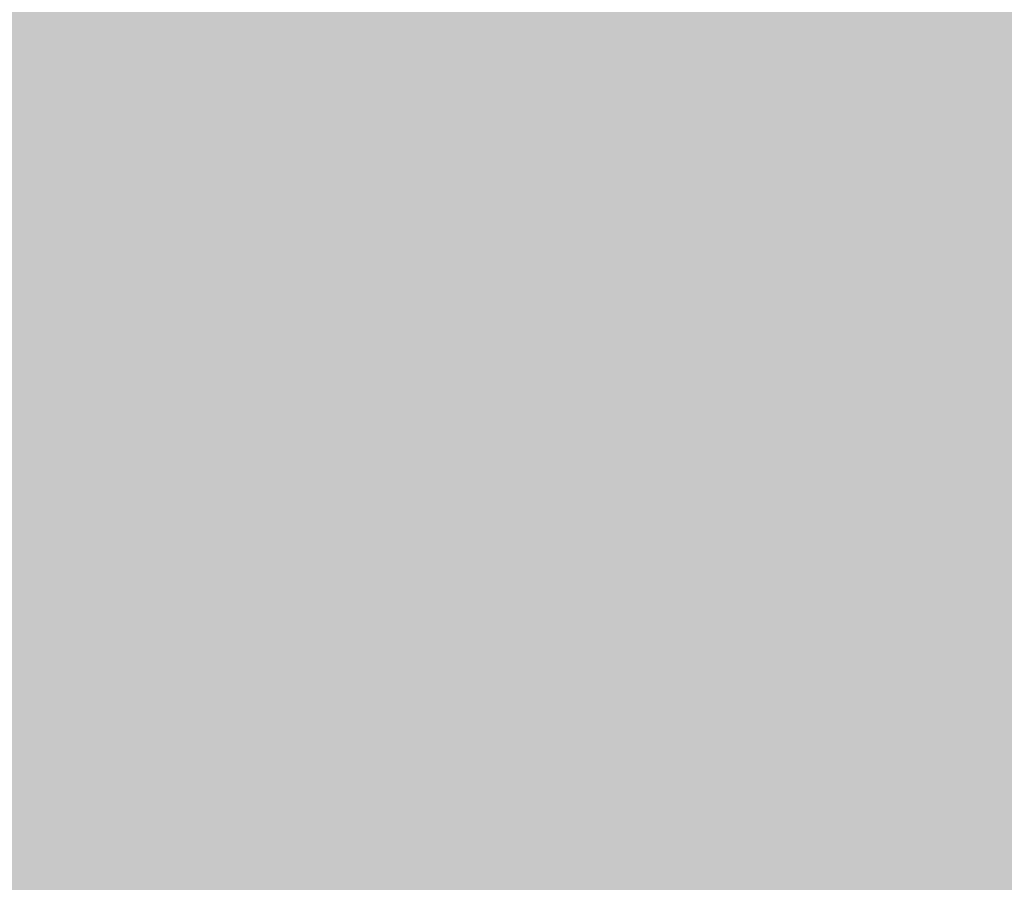
# Model space of a CAD drawing. Units: inches. Extents: x 2083 to 3317, y 1141 to 2115.
# Tile 149 of 256: x 3126.92826 to 3126.94671, y 1263.27402 to 1263.29018. Entities that reach past the tile are written whole.
import ezdxf

# ---------------------------------------------------------------- set-up
doc = ezdxf.new("R2010")
doc.units = ezdxf.units.IN
doc.layers.add('A-ANNO-DIMS', color=2, linetype='Continuous', lineweight=18)
doc.layers.add('A-WALL-PATT', color=251, linetype='Continuous', lineweight=13, true_color=0x636466)
doc.styles.get("Standard").update_dxf_attribs({"font": 'arial.ttf'})
doc.dimstyles.new('ISO-25', dxfattribs={"dimtxt": 12, "dimasz": 12, "dimexe": 1.25, "dimexo": 0.625, "dimtad": 1, "dimlunit": 3, "dimtxsty": 'Standard', "dimcen": 2.5, "dimadec": 0, "dimazin": 0, "dimtfac": 1, "dimtmove": 0, "dimatfit": 3, "dimfxl": 1, "dimarcsym": 0})

# ---------------------------------------------------------------- blocks, each defined once
blk = doc.blocks.new('*D26')
at = {"layer": 'A-ANNO-DIMS', "color": 0, "lineweight": -2, "transparency": 16777216}
for p, q in [((3088.985844, 1274.915092), (3088.985844, 1270.951963)), ((3111.240037, 1274.915092), (3111.240037, 1270.951963)), ((3076.985844, 1272.201963), (2840.262447, 1272.201963)), ((3111.240037, 1272.201963), (3088.985844, 1272.201963)), ((3123.240037, 1272.201963), (3135.240037, 1272.201963))]:
    blk.add_line(p, q, dxfattribs=at)
at = {"layer": 'A-ANNO-DIMS', "color": 0, "transparency": 16777216}
for points in [[(3076.985844, 1274.201963), (3076.985844, 1270.201963), (3088.985844, 1272.201963)], [(3123.240037, 1274.201963), (3123.240037, 1270.201963), (3111.240037, 1272.201963)]]:
    blk.add_solid(points, dxfattribs=at)
at = {"layer": 'Defpoints', "color": 0, "transparency": 16777216}
for p in [(3088.985844, 1275.540092), (3111.240037, 1275.540092), (3088.985844, 1272.201963)]:
    blk.add_point(p, dxfattribs=at)
at = {"layer": 'A-ANNO-DIMS', "color": 0, "transparency": 16777216, "insert": (2952.624146, 1279.031602), "char_height": 12, "attachment_point": 5}
blk.add_mtext('NIGHTSTAND 1\'-10 1/2" TYP.', dxfattribs=at)
blk = doc.blocks.new('*D27')
at = {"layer": 'A-ANNO-DIMS', "color": 0, "lineweight": -2, "transparency": 16777216}
for p, q in [((3114.578165, 1309.794285), (3114.578165, 1321.794285)), ((3111.865037, 1297.794285), (3115.828165, 1297.794285)), ((3114.578165, 1297.794285), (3114.578165, 1275.540092)), ((3111.865037, 1275.540092), (3115.828165, 1275.540092)), ((3114.578165, 1263.540092), (3114.578165, 1140.988591))]:
    blk.add_line(p, q, dxfattribs=at)
at = {"layer": 'A-ANNO-DIMS', "color": 0, "transparency": 16777216}
for points in [[(3112.578165, 1309.794285), (3116.578165, 1309.794285), (3114.578165, 1297.794285)], [(3112.578165, 1263.540092), (3116.578165, 1263.540092), (3114.578165, 1275.540092)]]:
    blk.add_solid(points, dxfattribs=at)
at = {"layer": 'Defpoints', "color": 0, "transparency": 16777216}
for p in [(3111.240037, 1297.794285), (3111.240037, 1275.540092), (3114.578165, 1275.540092)]:
    blk.add_point(p, dxfattribs=at)
at = {"layer": 'A-ANNO-DIMS', "color": 0, "transparency": 16777216, "insert": (3107.748527, 1196.264342), "char_height": 12, "attachment_point": 5, "rotation": 90}
blk.add_mtext('1\'-10 1/2" TYP.', dxfattribs=at)

msp = doc.modelspace()

# ---------------------------------------------------------------- hatches: boundary and pattern name
at = {"layer": 'A-WALL-PATT'}
h = msp.add_hatch(color=256, dxfattribs=at)
h.dxf.hatch_style = 1
h.paths.add_polyline_path([(3126.959783, 2020.76136), (2748.959783, 2020.76136), (2604.959783, 2020.76136), (2226.959783, 2020.76136), (2226.959783, 1702.76136), (2466.959783, 1702.76136), (2466.959783, 1582.76136), (2418.959783, 1582.76136), (2418.959783, 1477.76136), (2226.959783, 1477.76136), (2226.959783, 1263.26136), (2544.959783, 1263.26136), (2544.959783, 1411.76136), (2604.959783, 1411.76136), (2685.959783, 1411.76136), (2685.959783, 1420.76136), (2604.959783, 1420.76136), (2604.959783, 1573.76136), (2604.959783, 1702.76136), (2604.959783, 2011.76136), (2748.959783, 2011.76136), (2748.959783, 1702.76136), (2862.959783, 1702.76136), (2862.959783, 1621.76136), (2871.959783, 1621.76136), (2871.959783, 1702.76136), (2883.959783, 1702.76136), (2883.959783, 1706.939459, -0.026459), (2883.959783, 1711.76136), (2757.959783, 1711.76136), (2757.959783, 1807.76136), (2787.959783, 1807.76136), (2787.959783, 1812.26136), (2757.959783, 1812.26136), (2757.959783, 2011.76136), (2877.959783, 2011.76136), (2877.959783, 1812.26136), (2847.959783, 1812.26136), (2847.959783, 1807.76136), (2889.835742, 1807.76136), (2889.835742, 1812.26136), (2882.459783, 1812.26136), (2882.459783, 2011.76136), (3117.959783, 2011.76136), (3117.959783, 1812.26136), (2937.835742, 1812.26136), (2937.835742, 1807.76136), (2995.709783, 1807.76136), (2995.709783, 1796.117666), (3000.209783, 1796.117666), (3000.209783, 1807.76136), (3117.959783, 1807.76136), (3117.959783, 1711.76136), (3000.209783, 1711.76136), (3000.209783, 1760.117666), (2998.572705, 1760.117666, -0.020711), (2995.709783, 1760.117666), (2995.709783, 1711.76136), (2931.959783, 1711.76136), (2931.959783, 1702.76136), (3126.959783, 1702.76136)])
h.paths.add_polyline_path([(2471.459783, 2011.76136), (2471.459783, 1810.01136), (2462.716936, 1810.01136), (2462.716936, 1805.51136), (2505.959783, 1805.51136), (2505.959783, 1810.01136), (2475.959783, 1810.01136), (2475.959783, 2011.76136), (2595.959783, 2011.76136), (2595.959783, 1810.01136), (2565.959783, 1810.01136), (2565.959783, 1805.51136), (2595.959783, 1805.51136), (2595.959783, 1711.76136), (2235.959783, 1711.76136), (2235.959783, 1805.51136), (2353.709783, 1805.51136), (2353.709783, 1796.054162), (2358.209783, 1796.054162), (2358.209783, 1805.51136), (2414.716936, 1805.51136), (2414.716936, 1810.01136), (2235.959783, 1810.01136), (2235.959783, 2011.76136)], flags=16)
h.paths.add_polyline_path([(2270.204734, 1994.610008), (2270.204734, 1970.610008), (2246.204734, 1970.610008), (2246.204734, 1994.610008)], flags=0)
edge = h.paths.add_edge_path(flags=0)
edge.add_ellipse((2332.027391, 1899.798176), major_axis=(-3.042994, 3.042994), ratio=0.16825245, start_angle=-161.332166, end_angle=-156.307114, ccw=False)
edge.add_ellipse((2333.082037, 1898.74353), major_axis=(-1.054646, 1.054646), ratio=0.4535321, start_angle=-123.371019, end_angle=-94.159107)
edge = h.paths.add_edge_path(flags=0)
edge.add_ellipse((2332.027391, 1968.87629), major_axis=(3.042994, 3.042994), ratio=0.16825245, start_angle=18.667834, end_angle=23.692886)
edge.add_spline(control_points=[(2332.925596, 1970.691105), (2332.226768, 1970.3361), (2330.893709, 1969.658905), (2328.41308, 1970.932138), (2327.203934, 1967.748712), (2324.709596, 1969.955589), (2322.532822, 1967.012354), (2320.012846, 1971.295812), (2317.680308, 1968.157845), (2316.040526, 1967.102047), (2315.426904, 1966.809602)], knot_values=[0, 0, 0, 0, 2.267059, 4.324559, 6.685584, 8.878641, 11.121502, 14.300359, 17.755284, 19.732645, 19.732645, 19.732645, 19.732645], degree=3, periodic=0)
edge.add_ellipse((2332.027391, 1968.87629), major_axis=(3.042994, 3.042994), ratio=0.16825245, start_angle=18.667834, end_angle=23.692886, ccw=False)
edge.add_ellipse((2333.082037, 1969.930936), major_axis=(1.054646, 1.054646), ratio=0.4535321, start_angle=56.628981, end_angle=85.840893, ccw=False)
edge = h.paths.add_edge_path(flags=0)
edge.add_spline(control_points=[(2296.428287, 1967.987908), (2293.627804, 1965.336314), (2287.703624, 1959.727094), (2299.74386, 1949.995699), (2294.532591, 1935.668528), (2290.573228, 1920.603512), (2293.394124, 1909.973691), (2296.185407, 1904.966543)], knot_values=[0.099185, 0.099185, 0.099185, 0.099185, 0.345301, 0.619822, 0.982653, 1.386093, 1.810555, 1.810555, 1.810555, 1.810555], degree=3, periodic=0)
edge.add_spline(control_points=[(2296.185407, 1904.966543), (2297.383582, 1902.6193), (2298.000969, 1901.949312), (2298.55297, 1901.468155)], knot_values=[0.006246, 0.006246, 0.006246, 0.006246, 0.055476, 0.055476, 0.055476, 0.055476], degree=3, periodic=0)
edge.add_spline(control_points=[(2298.55297, 1901.468155), (2297.258612, 1900.923224), (2295.225294, 1900.232126), (2293.060229, 1900.614205), (2292.101423, 1900.788415), (2292.089578, 1900.790568)], knot_values=[0.312835, 0.312835, 0.312835, 0.312835, 0.40178, 0.474987, 0.475903, 0.475903, 0.475903, 0.475903], degree=3, periodic=0)
edge.add_arc((2292.793646, 1904.664109), 3.937008, 215.420897, 259.698179, ccw=False)
edge.add_spline(control_points=[(2289.585314, 1902.382304), (2289.476652, 1902.535087), (2289.36848, 1902.688035), (2289.260865, 1902.84117)], knot_values=[0.102872, 0.102872, 0.102872, 0.102872, 0.116896, 0.116896, 0.116896, 0.116896], degree=3, periodic=0)
edge.add_spline(control_points=[(2289.260865, 1902.84117), (2288.686604, 1902.550192), (2287.640048, 1902.019902), (2285.881337, 1901.873954), (2283.852972, 1901.504352), (2281.719987, 1899.710538), (2278.466991, 1899.492942), (2276.157136, 1901.883202), (2272.258953, 1899.804071), (2267.777605, 1901.843183), (2262.243882, 1900.184033), (2257.414927, 1901.782061), (2254.318374, 1900.72612), (2253.178285, 1900.337343)], knot_values=[0, 0, 0, 0, 1.907977, 3.477176, 5.261074, 7.972851, 11.680248, 13.717921, 16.939592, 22.789562, 27.502503, 33.595215, 37.145618, 37.145618, 37.145618, 37.145618], degree=3, periodic=0)
edge.add_line((2253.178285, 1900.337343), (2250.24424, 1902.84117))
edge.add_line((2250.24424, 1902.84117), (2250.24424, 1965.833296))
edge.add_line((2250.24424, 1965.833296), (2253.178285, 1968.337123))
edge.add_spline(control_points=[(2253.178285, 1968.337123), (2254.318374, 1967.948346), (2257.414927, 1966.892405), (2262.243882, 1968.490433), (2267.777605, 1966.831283), (2271.52673, 1968.537217), (2273.875914, 1967.828289), (2274.206701, 1967.727642)], knot_values=[0, 0, 0, 0, 0.09018, 0.244935, 0.364644, 0.513233, 0.537855, 0.537855, 0.537855, 0.537855], degree=3, periodic=0)
edge.add_arc((2274.352887, 1963.793349), 3.937008, 72.051134, 92.127949, ccw=False)
edge.add_arc((2281.296933, 1985.230003), 18.596298, 252.0511336, 288.5657217)
edge.add_arc((2292.316717, 1956.02888), 12.646081, 71.0267879, 113.7782184, ccw=False)
edge = h.paths.add_edge_path(flags=0)
edge.add_spline(control_points=[(2274.899415, 1951.856195), (2275.066156, 1951.616592), (2275.232687, 1951.376588), (2275.397987, 1951.135855)], knot_values=[1.409916, 1.409916, 1.409916, 1.409916, 1.43159, 1.43159, 1.43159, 1.43159], degree=3, periodic=0)
edge.add_spline(control_points=[(2275.397987, 1951.135855), (2275.792106, 1950.561885), (2276.179231, 1949.983774), (2276.545546, 1949.397103)], knot_values=[1.358238, 1.358238, 1.358238, 1.358238, 1.409916, 1.409916, 1.409916, 1.409916], degree=3, periodic=0)
edge.add_line((2276.545546, 1949.397103), (2277.437289, 1947.862185))
edge.add_spline(control_points=[(2277.437289, 1947.862185), (2276.303834, 1945.673115), (2274.639698, 1942.426882), (2274.631615, 1938.0939), (2272.799124, 1930.85155), (2274.356426, 1943.897046), (2275.947681, 1947.923356), (2276.545546, 1949.397103)], knot_values=[0.005632, 0.005632, 0.005632, 0.005632, 0.186014, 0.266002, 0.357087, 0.59639, 0.739732, 0.739732, 0.739732, 0.739732], degree=3, periodic=0)
edge.add_spline(control_points=[(2276.545546, 1949.397103), (2276.179231, 1949.983774), (2275.792106, 1950.561885), (2275.397987, 1951.135855)], knot_values=[1.358238, 1.358238, 1.358238, 1.358238, 1.409916, 1.409916, 1.409916, 1.409916], degree=3, periodic=0)
edge.add_spline(control_points=[(2275.397987, 1951.135855), (2274.9425, 1950.080452), (2274.20776, 1948.025272), (2273.934602, 1944.851477), (2272.468534, 1937.627489), (2273.466216, 1945.696466), (2274.700615, 1951.059472), (2274.899415, 1951.856195)], knot_values=[0.104364, 0.104364, 0.104364, 0.104364, 0.189636, 0.269624, 0.36071, 0.600013, 0.644622, 0.644622, 0.644622, 0.644622], degree=3, periodic=0)
h.paths.add_polyline_path([(2269.167514, 1963.127573, -0.357527), (2268.170633, 1960.97637, -0.092561), (2268.170633, 1939.436325, -0.357527), (2269.167514, 1937.285122, -0.357527), (2267.01631, 1938.282002, -0.164785), (2254.685581, 1938.282002, -0.357527), (2252.534378, 1937.285122, -0.357527), (2253.531259, 1939.436325, -0.092561), (2253.531259, 1960.97637, -0.357527), (2252.534378, 1963.127573, -0.357527), (2254.685581, 1962.130692, -0.164785), (2267.01631, 1962.130692, -0.357527)], flags=0)
h.paths.add_polyline_path([(2248.874068, 1967.8018), (2248.874068, 1957.02771), (2249.457783, 1957.02771), (2249.457783, 1911.646756), (2248.874068, 1911.646756), (2248.874068, 1900.872666), (2246.511863, 1900.872666, 0.197327), (2244.149658, 1902.456873), (2244.149658, 1966.217592, 0.197327), (2246.511863, 1967.8018)], flags=0)
h.paths.add_polyline_path([(2269.167514, 1931.389344, -0.357527), (2268.170633, 1929.238141, -0.092561), (2268.170633, 1907.698096, -0.357527), (2269.167514, 1905.546893, -0.357527), (2267.01631, 1906.543774, -0.164785), (2254.685581, 1906.543774, -0.357527), (2252.534378, 1905.546893, -0.357527), (2253.531259, 1907.698096, -0.092561), (2253.531259, 1929.238141, -0.357527), (2252.534378, 1931.389344, -0.357527), (2254.685581, 1930.392463, -0.164785), (2267.01631, 1930.392463, -0.357527)], flags=0)
edge = h.paths.add_edge_path(flags=0)
edge.add_spline(control_points=[(2276.196858, 1906.723702), (2276.168144, 1909.028928), (2276.114049, 1913.371852), (2270.598417, 1924.924978), (2273.905175, 1919.012779), (2275.921711, 1916.262063), (2275.47457, 1912.402149), (2277.257874, 1910.380621), (2276.696044, 1908.225036), (2276.646218, 1906.813023), (2276.617825, 1906.008407)], knot_values=[0, 0, 0, 0, 8.61026, 16.221274, 18.843057, 23.804898, 27.440828, 29.356102, 31.203478, 33.650687, 33.650687, 33.650687, 33.650687], degree=3, periodic=0)
edge.add_spline(control_points=[(2276.617825, 1906.008407), (2276.623313, 1905.624144), (2276.497738, 1904.628661), (2275.441779, 1903.854725), (2274.937314, 1903.08045), (2274.85908, 1902.84117)], knot_values=[0.156488, 0.156488, 0.156488, 0.156488, 0.184398, 0.231376, 0.250598, 0.250598, 0.250598, 0.250598], degree=3, periodic=0)
edge.add_line((2274.85908, 1902.84117), (2276.50598, 1902.84117))
edge.add_spline(control_points=[(2276.50598, 1902.84117), (2276.788308, 1903.08494), (2277.665071, 1904.125196), (2278.249538, 1904.340738), (2277.653872, 1908.527387), (2278.15567, 1906.227808), (2278.100464, 1905.285948), (2278.846675, 1904.069005), (2277.856785, 1903.414948), (2277.874191, 1902.99105), (2277.903562, 1902.84117)], knot_values=[0.059574, 0.059574, 0.059574, 0.059574, 0.080753, 0.103741, 0.16972, 0.176036, 0.207137, 0.240474, 0.262341, 0.27366, 0.27366, 0.27366, 0.27366], degree=3, periodic=0)
edge.add_line((2277.903562, 1902.84117), (2280.029825, 1902.84117))
edge.add_spline(control_points=[(2280.029825, 1902.84117), (2279.888221, 1903.088398), (2279.499257, 1903.981551), (2280.152284, 1905.939349), (2278.103615, 1909.657757), (2279.762395, 1907.185285), (2280.3279, 1904.874861), (2280.485109, 1903.48959), (2281.463269, 1903.249432), (2281.758343, 1902.936497), (2281.834036, 1902.84117)], knot_values=[0.013856, 0.013856, 0.013856, 0.013856, 0.034874, 0.088867, 0.107879, 0.126738, 0.158714, 0.193757, 0.217487, 0.226722, 0.226722, 0.226722, 0.226722], degree=3, periodic=0)
edge.add_spline(control_points=[(2281.834036, 1902.84117), (2281.787535, 1902.826703), (2281.647022, 1902.782988), (2281.395527, 1902.85949), (2281.088077, 1902.985242), (2280.720683, 1903.060902), (2280.333451, 1903.025726), (2280.124767, 1902.898879), (2280.029825, 1902.84117)], knot_values=[0, 0, 0, 0, 0.14413, 0.435517, 0.749276, 1.153046, 1.548371, 1.878348, 1.878348, 1.878348, 1.878348], degree=3, periodic=0)
edge.add_line((2280.029825, 1902.84117), (2277.903562, 1902.84117))
edge.add_spline(control_points=[(2277.903562, 1902.84117), (2277.892855, 1902.795855), (2277.865396, 1902.679637), (2277.607479, 1902.687483), (2277.27405, 1902.8007), (2276.837921, 1902.619775), (2276.583807, 1902.789261), (2276.50598, 1902.84117)], knot_values=[0, 0, 0, 0, 0.127189, 0.326199, 0.628009, 1.24357, 1.515331, 1.515331, 1.515331, 1.515331], degree=3, periodic=0)
edge.add_line((2276.50598, 1902.84117), (2274.85908, 1902.84117))
edge.add_spline(control_points=[(2274.85908, 1902.84117), (2274.814437, 1902.898587), (2274.72513, 1903.013446), (2274.493477, 1903.118968), (2274.244285, 1902.960539), (2273.937121, 1903.184942), (2273.614039, 1902.983143), (2273.408316, 1902.883045), (2273.322254, 1902.84117)], knot_values=[0, 0, 0, 0, 0.21843, 0.436957, 0.687977, 0.990379, 1.398396, 1.69185, 1.69185, 1.69185, 1.69185], degree=3, periodic=0)
edge.add_spline(control_points=[(2273.322254, 1902.84117), (2273.61674, 1903.445692), (2274.273998, 1904.538253), (2276.027239, 1904.573702), (2276.206963, 1906.583637), (2276.196858, 1906.723702)], knot_values=[0.012227, 0.012227, 0.012227, 0.012227, 0.059472, 0.106218, 0.134458, 0.134458, 0.134458, 0.134458], degree=3, periodic=0)
h.paths.add_polyline_path([(2270.776054, 1897.789828), (2270.776054, 1873.789828), (2246.776054, 1873.789828), (2246.776054, 1897.789828)], flags=0)
h.paths.add_polyline_path([(2353.709783, 1760.005059), (2353.709783, 1760.054162), (2358.209783, 1760.054162, -0.033729)], flags=0)
h.paths.add_polyline_path([(2321.819119, 1737.529186), (2341.995327, 1737.529186, -0.414214), (2343.203273, 1736.321241), (2343.203273, 1721.020596, -0.414214), (2341.995327, 1719.812651), (2321.819119, 1719.812651, -0.414214), (2320.611173, 1721.020596), (2320.611173, 1736.321241, -0.414214)], flags=0)
h.paths.add_polyline_path([(2324.23501, 1736.321241), (2339.579436, 1736.321241, -0.414214), (2341.995327, 1733.905349), (2341.995327, 1725.44973, -0.414214), (2339.579436, 1723.033839), (2333.680588, 1723.033839), (2333.845317, 1722.045467, -0.870646), (2335.425399, 1721.825893, -0.767327), (2333.922694, 1721.423245), (2331.291024, 1721.423245, -0.767327), (2329.788319, 1721.825893, -0.870646), (2331.368401, 1722.045467), (2331.53313, 1723.033839), (2324.23501, 1723.033839, -0.414214), (2321.819119, 1725.44973), (2321.819119, 1733.905349, -0.414214)], flags=0)
h.paths.add_polyline_path([(2570.483789, 1928.615444), (2589.683789, 1928.615444), (2590.168829, 1928.615444), (2590.168829, 1904.993397), (2570.483789, 1904.993397)], flags=0)
h.paths.add_polyline_path([(2574.447324, 1927.263822, -1), (2572.828836, 1927.263822, -1)], flags=0)
h.paths.add_polyline_path([(2573.089867, 1926.940877), (2573.925032, 1927.776042), (2574.147743, 1927.553332), (2573.312577, 1926.718166)], flags=0)
h.paths.add_polyline_path([(2578.779065, 1919.729618, -1), (2571.591663, 1919.729618, -1)], flags=0)
h.paths.add_polyline_path([(2578.385364, 1919.729618, -1), (2571.985364, 1919.729618, -1)], flags=0)
h.paths.add_polyline_path([(2331.595764, 1729.476216, -1), (2333.617954, 1729.476216, -1)], flags=0)
h.paths.add_polyline_path([(2578.034228, 1927.263822, -1), (2576.41574, 1927.263822, -1)], flags=0)
h.paths.add_polyline_path([(2576.688851, 1927.531089), (2576.911562, 1927.753799), (2577.746728, 1926.918634), (2577.524017, 1926.695923)], flags=0)
h.paths.add_polyline_path([(2578.139065, 1909.859539, -1), (2572.231663, 1909.859539, -1)], flags=0)
h.paths.add_polyline_path([(2577.745364, 1909.859539, -1), (2572.625364, 1909.859539, -1)], flags=0)
h.paths.add_polyline_path([(2583.797718, 1927.263822, -1), (2582.179229, 1927.263822, -1)], flags=0)
h.paths.add_polyline_path([(2582.718649, 1927.753799), (2583.553814, 1926.918634), (2583.331103, 1926.695923), (2582.495938, 1927.531089)], flags=0)
h.paths.add_polyline_path([(2582.495938, 1927.531089), (2582.718649, 1927.753799), (2583.553814, 1926.918634), (2583.331103, 1926.695923)], flags=0)
h.paths.add_polyline_path([(2587.739065, 1920.529618, -1), (2581.831663, 1920.529618, -1)], flags=0)
h.paths.add_polyline_path([(2587.345364, 1920.529618, -1), (2582.225364, 1920.529618, -1)], flags=0)
h.paths.add_polyline_path([(2587.384622, 1927.263822, -1), (2585.766133, 1927.263822, -1)], flags=0)
h.paths.add_polyline_path([(2586.081993, 1926.980247), (2586.917158, 1927.815412), (2587.139869, 1927.592702), (2586.304703, 1926.757536)], flags=0)
h.paths.add_polyline_path([(2588.379065, 1910.659539, -1), (2581.191663, 1910.659539, -1)], flags=0)
h.paths.add_polyline_path([(2587.985364, 1910.659539, -1), (2581.585364, 1910.659539, -1)], flags=0)
h.paths.add_polyline_path([(2417.167729, 1729.477895), (2437.343937, 1729.477895, -0.414214), (2438.551883, 1728.26995), (2438.551883, 1712.969306, -0.414214), (2437.343937, 1711.76136), (2417.167729, 1711.76136, -0.414214), (2415.959783, 1712.969306), (2415.959783, 1728.26995, -0.414214)], flags=0)
h.paths.add_polyline_path([(2419.58362, 1728.26995), (2434.928046, 1728.26995, -0.414214), (2437.343937, 1725.854059), (2437.343937, 1717.39844, -0.414214), (2434.928046, 1714.982548), (2429.029199, 1714.982548), (2429.193927, 1713.994176, -0.870646), (2430.774009, 1713.774603, -0.767327), (2429.271304, 1713.371954), (2426.639634, 1713.371954, -0.767327), (2425.136929, 1713.774603, -0.870646), (2426.717011, 1713.994176), (2426.88174, 1714.982548), (2419.58362, 1714.982548, -0.414214), (2417.167729, 1717.39844), (2417.167729, 1725.854059, -0.414214)], flags=0)
h.paths.add_polyline_path([(2419.58362, 1728.26995), (2434.928046, 1728.26995, -0.414214), (2437.343937, 1725.854059), (2437.343937, 1717.39844, -0.414214), (2434.928046, 1714.982548), (2429.029199, 1714.982548), (2428.358118, 1719.009034), (2427.552821, 1719.009034), (2426.88174, 1714.982548), (2419.58362, 1714.982548, -0.414214), (2417.167729, 1717.39844), (2417.167729, 1725.854059, -0.414214)], flags=0)
h.paths.add_polyline_path([(2426.944374, 1721.424925, -1), (2428.966564, 1721.424925, -1)], flags=0)
h.paths.add_polyline_path([(2475.959783, 1702.76136), (2595.959783, 1702.76136), (2595.959783, 1582.76136), (2475.959783, 1582.76136)], flags=16)
h.paths.add_polyline_path([(2427.959783, 1573.76136), (2595.959783, 1573.76136), (2595.959783, 1468.76136), (2595.959783, 1420.76136), (2384.459783, 1420.76136), (2384.459783, 1468.76136), (2427.959783, 1468.76136)], flags=16)
h.paths.add_polyline_path([(2379.959783, 1468.76136), (2379.959783, 1420.76136), (2235.959783, 1420.76136), (2235.959783, 1468.76136)], flags=16)
h.paths.add_polyline_path([(2317.815996, 1466.695767), (2337.992205, 1466.695767, -0.414214), (2339.20015, 1465.487821), (2339.20015, 1450.187177, -0.414214), (2337.992205, 1448.979232), (2317.815996, 1448.979232, -0.414214), (2316.608051, 1450.187177), (2316.608051, 1465.487821, -0.414214)], flags=0)
h.paths.add_polyline_path([(2320.231887, 1465.487821), (2335.576313, 1465.487821, -0.414214), (2337.992205, 1463.07193), (2337.992205, 1454.616311, -0.414214), (2335.576313, 1452.20042), (2329.677466, 1452.20042), (2329.842195, 1451.212047, -0.870646), (2331.422276, 1450.992474, -0.767327), (2329.919571, 1450.589826), (2327.287902, 1450.589826, -0.767327), (2325.785197, 1450.992474, -0.870646), (2327.365278, 1451.212047), (2327.530007, 1452.20042), (2320.231887, 1452.20042, -0.414214), (2317.815996, 1454.616311), (2317.815996, 1463.07193, -0.414214)], flags=0)
h.paths.add_polyline_path([(2320.231887, 1465.487821), (2335.576313, 1465.487821, -0.414214), (2337.992205, 1463.07193), (2337.992205, 1454.616311, -0.414214), (2335.576313, 1452.20042), (2329.677466, 1452.20042), (2329.006385, 1456.226905), (2328.201088, 1456.226905), (2327.530007, 1452.20042), (2320.231887, 1452.20042, -0.414214), (2317.815996, 1454.616311), (2317.815996, 1463.07193, -0.414214)], flags=0)
h.paths.add_polyline_path([(2327.592641, 1458.642796, -1), (2329.614832, 1458.642796, -1)], flags=0)
h.paths.add_polyline_path([(2244.411744, 1433.340453), (2241.920945, 1433.340453, -0.414214), (2240.017856, 1435.243542), (2240.017856, 1440.952808, -0.414211), (2241.920925, 1442.855897), (2244.411744, 1442.855897, -1.976472)], flags=0)
h.paths.add_polyline_path([(2245.356888, 1434.397536, -0.414214), (2245.356888, 1441.798814, -2.144098)], flags=0)
h.paths.add_polyline_path([(2535.959783, 1416.26136), (2535.959783, 1272.26136), (2235.959783, 1272.26136), (2235.959783, 1416.26136)], flags=16)
h.paths.add_polyline_path([(2260.119561, 1384.292841), (2260.119561, 1362.038649), (2237.865369, 1362.038649), (2237.865369, 1384.292841)], flags=0)
edge = h.paths.add_edge_path(flags=0)
edge.add_line((2318.251847, 1362.093298), (2318.145797, 1362.000973))
edge.add_ellipse((2317.445116, 1360.431044), major_axis=(2.82164, 2.82164), ratio=0.16825245, start_angle=18.667834, end_angle=20.948127, ccw=False)
edge.add_ellipse((2318.423045, 1361.408974), major_axis=(0.977929, 0.977929), ratio=0.4535321, start_angle=56.628981, end_angle=70.226201, ccw=False)
edge = h.paths.add_edge_path(flags=0)
edge.add_line((2319.10737, 1295.571078), (2319.015044, 1295.677128))
edge.add_ellipse((2317.445116, 1296.377809), major_axis=(-2.82164, 2.82164), ratio=0.16825245, start_angle=-161.332166, end_angle=-159.051873, ccw=False)
edge.add_ellipse((2318.423045, 1295.39988), major_axis=(-0.977929, 0.977929), ratio=0.4535321, start_angle=-123.371019, end_angle=-109.773799)
edge = h.paths.add_edge_path(flags=0)
edge.add_spline(control_points=[(2284.210349, 1301.170219), (2284.580688, 1300.444719), (2284.891189, 1299.892024), (2285.159553, 1299.461018)], knot_values=[0.039066, 0.039066, 0.039066, 0.039066, 0.055476, 0.055476, 0.055476, 0.055476], degree=3, periodic=0)
edge.add_line((2285.159553, 1299.461018), (2284.210349, 1301.170219))
edge = h.paths.add_edge_path(flags=0)
edge.add_line((2280.412458, 1297.298013), (2283.369991, 1297.036122))
edge.add_line((2283.369991, 1297.036122), (2286.40569, 1297.92631))
edge.add_spline(control_points=[(2286.40569, 1297.92631), (2285.305487, 1297.463119), (2284.344777, 1297.129151), (2283.369991, 1297.036122)], knot_values=[0.394369, 0.394369, 0.394369, 0.394369, 0.475903, 0.475903, 0.475903, 0.475903], degree=3, periodic=0)
edge.add_spline(control_points=[(2283.369991, 1297.036122), (2283.28139, 1297.027666), (2282.316289, 1296.957336), (2281.312502, 1297.134479), (2280.423441, 1297.296016), (2280.412458, 1297.298013)], knot_values=[0.312835, 0.312835, 0.312835, 0.312835, 0.320246, 0.393453, 0.394369, 0.394369, 0.394369, 0.394369], degree=3, periodic=0)
edge = h.paths.add_edge_path(flags=0)
edge.add_line((2284.435561, 1359.607285), (2280.446291, 1355.328047))
edge.add_line((2280.446291, 1355.328047), (2279.579987, 1351.017754))
edge.add_line((2279.579987, 1351.017754), (2282.412974, 1346.580433))
edge.add_spline(control_points=[(2282.412974, 1346.580433), (2283.153331, 1345.589236), (2284.252896, 1344.028897), (2284.801037, 1342.387167), (2284.935162, 1341.805544)], knot_values=[1.240098, 1.240098, 1.240098, 1.240098, 1.332892, 1.382712, 1.382712, 1.382712, 1.382712], degree=3, periodic=0)
edge.add_spline(control_points=[(2284.935162, 1341.805544), (2285.319108, 1340.1406), (2285.233029, 1338.409204), (2284.909938, 1336.654122)], knot_values=[1.097484, 1.097484, 1.097484, 1.097484, 1.240098, 1.240098, 1.240098, 1.240098], degree=3, periodic=0)
edge.add_spline(control_points=[(2284.909938, 1336.654122), (2284.586848, 1334.89904), (2284.026745, 1333.120272), (2283.462644, 1331.360585)], knot_values=[0.95487, 0.95487, 0.95487, 0.95487, 1.097484, 1.097484, 1.097484, 1.097484], degree=3, periodic=0)
edge.add_line((2283.462644, 1331.360585), (2281.890376, 1326.153357))
edge.add_line((2281.890376, 1326.153357), (2280.756259, 1321.056089))
edge.add_line((2280.756259, 1321.056089), (2280.299205, 1316.001977))
edge.add_line((2280.299205, 1316.001977), (2280.715933, 1310.950068))
edge.add_line((2280.715933, 1310.950068), (2282.028094, 1305.972137))
edge.add_line((2282.028094, 1305.972137), (2284.210349, 1301.170219))
edge.add_spline(control_points=[(2284.210349, 1301.170219), (2283.340731, 1302.730185), (2282.611904, 1304.336493), (2282.028094, 1305.972137)], knot_values=[0.099185, 0.099185, 0.099185, 0.099185, 0.241799, 0.241799, 0.241799, 0.241799], degree=3, periodic=0)
edge.add_spline(control_points=[(2282.028094, 1305.972137), (2281.444283, 1307.60778), (2281.005489, 1309.272759), (2280.715933, 1310.950068)], knot_values=[0.241799, 0.241799, 0.241799, 0.241799, 0.384413, 0.384413, 0.384413, 0.384413], degree=3, periodic=0)
edge.add_spline(control_points=[(2280.715933, 1310.950068), (2280.433241, 1312.587613), (2280.289386, 1314.276959), (2280.298894, 1315.962032), (2280.299205, 1316.001977)], knot_values=[0.384413, 0.384413, 0.384413, 0.384413, 0.523647, 0.527028, 0.527028, 0.527028, 0.527028], degree=3, periodic=0)
edge.add_spline(control_points=[(2280.299205, 1316.001977), (2280.312326, 1317.686955), (2280.477871, 1319.367926), (2280.756259, 1321.056089)], knot_values=[0.527028, 0.527028, 0.527028, 0.527028, 0.669642, 0.669642, 0.669642, 0.669642], degree=3, periodic=0)
edge.add_spline(control_points=[(2280.756259, 1321.056089), (2281.034648, 1322.744252), (2281.42588, 1324.439608), (2281.890376, 1326.153357)], knot_values=[0.669642, 0.669642, 0.669642, 0.669642, 0.812256, 0.812256, 0.812256, 0.812256], degree=3, periodic=0)
edge.add_spline(control_points=[(2281.890376, 1326.153357), (2282.264383, 1327.533251), (2282.78787, 1329.26181), (2283.352751, 1331.01778), (2283.462644, 1331.360585)], knot_values=[0.812256, 0.812256, 0.812256, 0.812256, 0.927087, 0.95487, 0.95487, 0.95487, 0.95487], degree=3, periodic=0)
edge.add_line((2283.462644, 1331.360585), (2284.909938, 1336.654122))
edge.add_line((2284.909938, 1336.654122), (2284.935162, 1341.805544))
edge.add_line((2284.935162, 1341.805544), (2282.412974, 1346.580433))
edge.add_spline(control_points=[(2282.412974, 1346.580433), (2281.275127, 1348.103792), (2280.078447, 1349.570318), (2279.579987, 1351.017754)], knot_values=[1.382712, 1.382712, 1.382712, 1.382712, 1.525326, 1.525326, 1.525326, 1.525326], degree=3, periodic=0)
edge.add_spline(control_points=[(2279.579987, 1351.017754), (2279.443282, 1351.414721), (2279.136312, 1352.856922), (2279.73519, 1354.290385), (2280.446291, 1355.328047)], knot_values=[1.525326, 1.525326, 1.525326, 1.525326, 1.564439, 1.667941, 1.667941, 1.667941, 1.667941], degree=3, periodic=0)
edge.add_spline(control_points=[(2280.446291, 1355.328047), (2281.426113, 1356.757835), (2282.930837, 1358.18256), (2284.435561, 1359.607285)], knot_values=[1.667941, 1.667941, 1.667941, 1.667941, 1.810555, 1.810555, 1.810555, 1.810555], degree=3, periodic=0)
edge.add_arc((2280.623075, 1348.518181), 11.72618, 71.0267879, 113.7782184)
edge.add_arc((2270.404892, 1375.595156), 17.243567, 252.0511336, 288.5657217, ccw=False)
edge.add_arc((2263.965969, 1355.717847), 3.650622, 72.051134, 92.127949)
edge.add_arc((2263.965969, 1355.717847), 3.650622, 92.127949, 177.98513)
edge.add_spline(control_points=[(2260.317604, 1355.846199), (2260.260417, 1354.220668), (2260.551278, 1350.186547), (2262.999344, 1346.766251), (2264.472741, 1344.649024)], knot_values=[1.43159, 1.43159, 1.43159, 1.43159, 1.564144, 1.770695, 1.770695, 1.770695, 1.770695], degree=3, periodic=0)
edge.add_line((2264.472741, 1344.649024), (2264.93559, 1343.98253))
edge.add_spline(control_points=[(2263.801044, 1340.248105), (2263.843238, 1340.514088), (2264.067244, 1341.756465), (2264.512693, 1343.002453), (2264.935047, 1343.981083)], knot_values=[0.53657, 0.53657, 0.53657, 0.53657, 0.559349, 0.644622, 0.644622, 0.644622, 0.644622], degree=3, periodic=0)
edge.add_spline(control_points=[(2264.935047, 1343.981083), (2265.117771, 1343.714975), (2265.298875, 1343.447906), (2265.476756, 1343.179365)], knot_values=[1.384077, 1.384077, 1.384077, 1.384077, 1.409916, 1.409916, 1.409916, 1.409916], degree=3, periodic=0)
edge.add_spline(control_points=[(2265.476756, 1343.179365), (2265.654637, 1342.910823), (2265.829296, 1342.64081), (2265.99913, 1342.368812)], knot_values=[1.358238, 1.358238, 1.358238, 1.358238, 1.384077, 1.384077, 1.384077, 1.384077], degree=3, periodic=0)
edge.add_line((2265.99913, 1342.368812), (2266.826006, 1340.945547))
edge.add_spline(control_points=[(2266.826006, 1340.945547), (2268.894401, 1337.089691), (2271.398173, 1325.843001), (2270.516164, 1310.568557), (2275.919376, 1301.860609), (2277.789511, 1299.19945)], knot_values=[0.116896, 0.116896, 0.116896, 0.116896, 0.472987, 1.050969, 1.313793, 1.313793, 1.313793, 1.313793], degree=3, periodic=0)
edge.add_spline(control_points=[(2277.789511, 1299.19945), (2277.839405, 1299.128452), (2277.889428, 1299.057498), (2277.939572, 1298.986584)], knot_values=[0.109884, 0.109884, 0.109884, 0.109884, 0.116896, 0.116896, 0.116896, 0.116896], degree=3, periodic=0)
edge.add_line((2277.939572, 1298.986584), (2277.788849, 1299.199114))
edge.add_spline(control_points=[(2277.788849, 1299.199114), (2277.256582, 1298.929414), (2276.28635, 1298.437902), (2275.039352, 1298.334419), (2274.38333, 1298.238895), (2274.215254, 1298.209338)], knot_values=[33.12187, 33.12187, 33.12187, 33.12187, 35.029056, 36.598255, 37.144827, 37.144827, 37.144827, 37.144827], degree=3, periodic=0)
edge.add_line((2274.215254, 1298.209338), (2273.073147, 1297.892961))
edge.add_spline(control_points=[(2273.073147, 1297.892961), (2272.322936, 1297.579784), (2271.039151, 1296.510508), (2269.248395, 1296.226062), (2268.4231, 1296.374654)], knot_values=[26.532584, 26.532584, 26.532584, 26.532584, 29.198919, 31.839101, 31.839101, 31.839101, 31.839101], degree=3, periodic=0)
edge.add_line((2268.4231, 1296.374654), (2263.878501, 1297.457534))
edge.add_spline(control_points=[(2263.878501, 1297.457534), (2263.556077, 1297.359435), (2261.860306, 1296.838694), (2260.23878, 1297.282407), (2258.933454, 1297.516461)], knot_values=[15.919551, 15.919551, 15.919551, 15.919551, 16.939592, 21.226067, 21.226067, 21.226067, 21.226067], degree=3, periodic=0)
edge.add_line((2258.933454, 1297.516461), (2254.055233, 1297.32901))
edge.add_spline(control_points=[(2254.055233, 1297.32901), (2253.755525, 1297.295815), (2252.113683, 1297.165174), (2250.461869, 1297.544221), (2249.129686, 1297.667882)], knot_values=[5.306517, 5.306517, 5.306517, 5.306517, 6.276435, 10.613034, 10.613034, 10.613034, 10.613034], degree=3, periodic=0)
edge.add_line((2249.129686, 1297.667882), (2244.33165, 1296.877756))
edge.add_line((2244.33165, 1296.877756), (2241.611033, 1299.19945))
edge.add_line((2241.611033, 1299.19945), (2241.611033, 1357.609404))
edge.add_line((2241.611033, 1357.609404), (2244.33165, 1359.931097))
edge.add_line((2244.33165, 1359.931097), (2252.728823, 1359.542692))
edge.add_spline(control_points=[(2252.728823, 1359.542692), (2252.870939, 1359.54644), (2253.30574, 1359.548172), (2253.739845, 1359.514274), (2254.031742, 1359.482426)], knot_values=[0.233291, 0.233291, 0.233291, 0.233291, 0.244935, 0.268927, 0.268927, 0.268927, 0.268927], degree=3, periodic=0)
edge.add_line((2254.031742, 1359.482426), (2259.58719, 1359.41639))
edge.add_spline(control_points=[(2259.58719, 1359.41639), (2260.677068, 1359.628503), (2262.073197, 1359.897003), (2263.523692, 1359.459278), (2263.830417, 1359.365952)], knot_values=[0.422516, 0.422516, 0.422516, 0.422516, 0.513233, 0.537855, 0.537855, 0.537855, 0.537855], degree=3, periodic=0)
edge.add_arc((2263.965969, 1355.717847), 3.650622, 72.051134, 92.127949, ccw=False)
edge.add_arc((2270.404892, 1375.595156), 17.243567, 252.0511336, 288.5657217)
edge.add_arc((2280.623075, 1348.518181), 11.72618, 71.0267879, 113.7782184, ccw=False)
h.paths.add_polyline_path([(2240.34053, 1359.434715), (2240.34053, 1349.444353), (2240.881785, 1349.444353), (2240.881785, 1307.3645), (2240.34053, 1307.3645), (2240.34053, 1297.374138), (2238.150157, 1297.374138, 0.197327), (2235.959783, 1298.843108), (2235.959783, 1357.965746, 0.197327), (2238.150157, 1359.434715)], flags=0)
h.paths.add_polyline_path([(2259.15779, 1355.1005, -0.357527), (2258.233425, 1353.10578, -0.092561), (2258.233425, 1333.132601, -0.357527), (2259.15779, 1331.13788, -0.357527), (2257.16307, 1332.062246, -0.164785), (2245.729302, 1332.062246, -0.357527), (2243.734582, 1331.13788, -0.357527), (2244.658947, 1333.132601, -0.092561), (2244.658947, 1353.10578, -0.357527), (2243.734582, 1355.1005, -0.357527), (2245.729302, 1354.176135, -0.164785), (2257.16307, 1354.176135, -0.357527)], flags=0)
edge = h.paths.add_edge_path(flags=0)
edge.add_line((2265.99913, 1342.368812), (2266.826006, 1340.945547))
edge.add_line((2266.826006, 1340.945547), (2265.307557, 1337.814066))
edge.add_line((2265.307557, 1337.814066), (2264.358232, 1334.652939))
edge.add_line((2264.358232, 1334.652939), (2264.262012, 1333.799705))
edge.add_spline(control_points=[(2264.262012, 1333.799705), (2264.208357, 1333.187055), (2264.16206, 1332.365525), (2264.007144, 1331.413933), (2263.969049, 1331.201834)], knot_values=[0.464444, 0.464444, 0.464444, 0.464444, 0.516691, 0.531608, 0.531608, 0.531608, 0.531608], degree=3, periodic=0)
edge.add_spline(control_points=[(2263.969049, 1331.201834), (2263.774535, 1330.118873), (2263.42437, 1328.790839), (2263.25742, 1328.530652), (2263.234028, 1328.514612)], knot_values=[0.372682, 0.372682, 0.372682, 0.372682, 0.44885, 0.464444, 0.464444, 0.464444, 0.464444], degree=3, periodic=0)
edge.add_spline(control_points=[(2263.234028, 1328.514612), (2263.096382, 1328.420227), (2263.13117, 1329.301477), (2263.274953, 1330.615749)], knot_values=[0.280919, 0.280919, 0.280919, 0.280919, 0.372682, 0.372682, 0.372682, 0.372682], degree=3, periodic=0)
edge.add_spline(control_points=[(2263.274953, 1330.615749), (2263.418736, 1331.930022), (2263.671515, 1333.677318), (2263.969852, 1335.315027)], knot_values=[0.189157, 0.189157, 0.189157, 0.189157, 0.280919, 0.280919, 0.280919, 0.280919], degree=3, periodic=0)
edge.add_spline(control_points=[(2263.969852, 1335.315027), (2264.100496, 1336.032192), (2264.418783, 1337.621911), (2264.754848, 1338.86443), (2264.947419, 1339.491124)], knot_values=[0.097394, 0.097394, 0.097394, 0.097394, 0.137578, 0.189157, 0.189157, 0.189157, 0.189157], degree=3, periodic=0)
edge.add_spline(control_points=[(2264.947419, 1339.491124), (2265.290017, 1340.606055), (2265.644238, 1341.493996), (2265.99913, 1342.368812)], knot_values=[0.005632, 0.005632, 0.005632, 0.005632, 0.097394, 0.097394, 0.097394, 0.097394], degree=3, periodic=0)
h.paths.add_polyline_path([(2259.15779, 1325.670973, -0.357527), (2258.233425, 1323.676253, -0.092561), (2258.233425, 1303.703073, -0.357527), (2259.15779, 1301.708353, -0.357527), (2257.16307, 1302.632719, -0.164785), (2245.729302, 1302.632719, -0.357527), (2243.734582, 1301.708353, -0.357527), (2244.658947, 1303.703073, -0.092561), (2244.658947, 1323.676253, -0.357527), (2243.734582, 1325.670973, -0.357527), (2245.729302, 1324.746608, -0.164785), (2257.16307, 1324.746608, -0.357527)], flags=0)
edge = h.paths.add_edge_path(flags=0)
edge.add_spline(control_points=[(2261.708938, 1317.311421), (2261.679482, 1317.41758), (2261.761858, 1317.388535), (2262.490736, 1316.089873), (2262.962185, 1315.300897)], knot_values=[14.955861, 14.955861, 14.955861, 14.955861, 16.221274, 18.694826, 18.694826, 18.694826, 18.694826], degree=3, periodic=0)
edge.add_spline(control_points=[(2262.962185, 1315.300897), (2262.990437, 1315.253617), (2263.702096, 1314.067376), (2264.348983, 1313.127153), (2264.730054, 1312.164154)], knot_values=[18.694826, 18.694826, 18.694826, 18.694826, 18.843057, 22.433791, 22.433791, 22.433791, 22.433791], degree=3, periodic=0)
edge.add_spline(control_points=[(2264.730054, 1312.164154), (2264.875565, 1311.796437), (2265.176873, 1310.769807), (2265.143069, 1309.559262), (2265.247736, 1308.824193)], knot_values=[22.433791, 22.433791, 22.433791, 22.433791, 23.804898, 26.172756, 26.172756, 26.172756, 26.172756], degree=3, periodic=0)
edge.add_line((2265.247736, 1308.824193), (2265.850774, 1307.171888))
edge.add_spline(control_points=[(2265.850774, 1307.171888), (2266.065025, 1306.821678), (2266.384387, 1306.332246), (2266.4244, 1305.780549), (2266.420369, 1305.611216)], knot_values=[28.062562, 28.062562, 28.062562, 28.062562, 29.356102, 29.911721, 29.911721, 29.911721, 29.911721], degree=3, periodic=0)
edge.add_spline(control_points=[(2266.420369, 1305.611216), (2266.416116, 1305.43259), (2266.393999, 1305.249998), (2266.364777, 1305.065857)], knot_values=[29.911721, 29.911721, 29.911721, 29.911721, 30.497837, 30.497837, 30.497837, 30.497837], degree=3, periodic=0)
edge.add_line((2266.364777, 1305.065857), (2266.066151, 1302.136295))
edge.add_spline(control_points=[(2266.066151, 1302.136295), (2266.07124, 1301.779984), (2265.998076, 1301.199985), (2265.663266, 1300.758961), (2265.508908, 1300.585882)], knot_values=[0.156488, 0.156488, 0.156488, 0.156488, 0.184398, 0.203543, 0.203543, 0.203543, 0.203543], degree=3, periodic=0)
edge.add_line((2265.508908, 1300.585882), (2264.435341, 1299.19945))
edge.add_line((2264.435341, 1299.19945), (2265.962442, 1299.19945))
edge.add_line((2265.962442, 1299.19945), (2267.33599, 1301.175276))
edge.add_line((2267.33599, 1301.175276), (2267.311667, 1301.986237))
edge.add_spline(control_points=[(2267.311667, 1301.986237), (2267.261111, 1302.862396), (2267.160212, 1303.737132), (2267.271486, 1303.325896)], knot_values=[0.126229, 0.126229, 0.126229, 0.126229, 0.166617, 0.166617, 0.166617, 0.166617], degree=3, periodic=0)
edge.add_spline(control_points=[(2267.271486, 1303.325896), (2267.280035, 1303.294305), (2267.309785, 1303.175366), (2267.37345, 1302.883608), (2267.406123, 1302.682829), (2267.417926, 1302.601025)], knot_values=[0.166617, 0.166617, 0.166617, 0.166617, 0.16972, 0.176036, 0.180765, 0.180765, 0.180765, 0.180765], degree=3, periodic=0)
edge.add_spline(control_points=[(2267.743891, 1300.987505), (2267.687583, 1301.150943), (2267.48052, 1301.656664), (2267.483751, 1302.144788), (2267.417926, 1302.601025)], knot_values=[0.180765, 0.180765, 0.180765, 0.180765, 0.193767, 0.220139, 0.220139, 0.220139, 0.220139], degree=3, periodic=0)
edge.add_line((2267.417926, 1302.601025), (2267.743891, 1300.987505))
edge.add_spline(control_points=[(2267.743891, 1300.987505), (2267.831961, 1300.731878), (2267.932021, 1300.309904), (2267.554841, 1299.974518), (2267.429366, 1299.829207)], knot_values=[0.220139, 0.220139, 0.220139, 0.220139, 0.240474, 0.25489, 0.25489, 0.25489, 0.25489], degree=3, periodic=0)
edge.add_line((2267.429366, 1299.829207), (2267.258361, 1299.19945))
edge.add_line((2267.258361, 1299.19945), (2269.229956, 1299.19945))
edge.add_spline(control_points=[(2269.229956, 1299.19945), (2269.098653, 1299.428694), (2268.842774, 1300.016251), (2269.011575, 1300.915923), (2268.946796, 1301.66074)], knot_values=[0.013856, 0.013856, 0.013856, 0.013856, 0.034874, 0.067073, 0.067073, 0.067073, 0.067073], degree=3, periodic=0)
edge.add_line((2268.946796, 1301.66074), (2268.431582, 1303.603109))
edge.add_spline(control_points=[(2268.431582, 1303.603109), (2268.175596, 1304.192375), (2267.596214, 1305.251298), (2268.040698, 1304.62321), (2268.251394, 1304.282421)], knot_values=[0.090155, 0.090155, 0.090155, 0.090155, 0.107879, 0.120289, 0.120289, 0.120289, 0.120289], degree=3, periodic=0)
edge.add_spline(control_points=[(2268.251394, 1304.282421), (2268.360882, 1304.105329), (2269.057753, 1302.917983), (2269.382691, 1301.590419), (2269.521405, 1300.775931), (2269.57522, 1300.555784)], knot_values=[0.120289, 0.120289, 0.120289, 0.120289, 0.126738, 0.158714, 0.173506, 0.173506, 0.173506, 0.173506], degree=3, periodic=0)
edge.add_line((2269.57522, 1300.555784), (2270.685798, 1299.421258))
edge.add_spline(control_points=[(2270.685798, 1299.421258), (2270.767221, 1299.357251), (2270.837852, 1299.281401), (2270.902925, 1299.19945)], knot_values=[0.21816, 0.21816, 0.21816, 0.21816, 0.226722, 0.226722, 0.226722, 0.226722], degree=3, periodic=0)
edge.add_line((2270.937201, 1299.192913), (2270.902925, 1299.19945))
edge.add_spline(control_points=[(2270.902925, 1299.19945), (2270.859806, 1299.186035), (2270.729515, 1299.1455), (2270.496314, 1299.216437), (2270.271661, 1299.308323), (2270.121017, 1299.347961), (2270.063339, 1299.359557)], knot_values=[0.939174, 0.939174, 0.939174, 0.939174, 1.083304, 1.374691, 1.68845, 1.878348, 1.878348, 1.878348, 1.878348], degree=3, periodic=0)
edge.add_line((2270.063339, 1299.359557), (2269.229956, 1299.19945))
edge.add_line((2269.229956, 1299.19945), (2267.258361, 1299.19945))
edge.add_spline(control_points=[(2267.258361, 1299.19945), (2267.248433, 1299.157431), (2267.222971, 1299.049667), (2266.983816, 1299.056942), (2266.80921, 1299.11623), (2266.676905, 1299.109091), (2266.636531, 1299.104815)], knot_values=[0.757665, 0.757665, 0.757665, 0.757665, 0.884854, 1.083864, 1.385675, 1.515331, 1.515331, 1.515331, 1.515331], degree=3, periodic=0)
edge.add_spline(control_points=[(2266.636531, 1299.104815), (2266.485225, 1299.088788), (2266.235807, 1299.017123), (2266.034608, 1299.151317), (2265.962442, 1299.19945)], knot_values=[0, 0, 0, 0, 0.485905, 0.757665, 0.757665, 0.757665, 0.757665], degree=3, periodic=0)
edge.add_line((2265.962442, 1299.19945), (2264.435341, 1299.19945))
edge.add_line((2264.435341, 1299.19945), (2263.858444, 1299.367118))
edge.add_spline(control_points=[(2263.858444, 1299.367118), (2263.818943, 1299.370905), (2263.779528, 1299.385721), (2263.740131, 1299.401504)], knot_values=[0.845925, 0.845925, 0.845925, 0.845925, 0.978627, 0.978627, 0.978627, 0.978627], degree=3, periodic=0)
edge.add_line((2263.721786, 1299.396425), (2263.010306, 1299.19945))
edge.add_spline(control_points=[(2263.010306, 1299.19945), (2263.245794, 1299.682859), (2263.506032, 1300.128107), (2263.873494, 1300.408028)], knot_values=[0.012227, 0.012227, 0.012227, 0.012227, 0.052971, 0.052971, 0.052971, 0.052971], degree=3, periodic=0)
edge.add_spline(control_points=[(2263.873494, 1300.408028), (2263.932131, 1300.452695), (2264.084243, 1300.552979), (2264.255189, 1300.624223), (2264.359686, 1300.664747)], knot_values=[0.052971, 0.052971, 0.052971, 0.052971, 0.059472, 0.069086, 0.069086, 0.069086, 0.069086], degree=3, periodic=0)
edge.add_line((2264.359686, 1300.664747), (2265.1419, 1301.077774))
edge.add_line((2265.1419, 1301.077774), (2265.675806, 1302.799558))
edge.add_line((2265.675806, 1302.799558), (2265.5407, 1305.704066))
edge.add_line((2265.5407, 1305.704066), (2264.803073, 1309.327724))
edge.add_line((2264.803073, 1309.327724), (2263.040535, 1314.091791))
edge.add_spline(control_points=[(2263.040535, 1314.091791), (2262.383572, 1315.671438), (2261.795972, 1316.997749), (2261.708938, 1317.311421)], knot_values=[11.216896, 11.216896, 11.216896, 11.216896, 14.955861, 14.955861, 14.955861, 14.955861], degree=3, periodic=0)
h.paths.add_polyline_path([(2871.959783, 1416.26136), (2895.910047, 1416.26136), (2895.910047, 1420.76136), (2871.959783, 1420.76136), (2871.959783, 1501.76136), (2862.959783, 1501.76136), (2862.959783, 1420.76136), (2805.959783, 1420.76136), (2805.959783, 1411.76136), (2862.959783, 1411.76136), (2862.959783, 1263.26136), (3126.959783, 1263.26136), (3126.959783, 1411.76136), (3126.959783, 1486.76136), (2943.959783, 1486.76136), (2943.959783, 1477.76136), (2967.860311, 1477.76136), (2967.860311, 1420.76136), (2943.910047, 1420.76136), (2943.910047, 1416.26136), (3117.959783, 1416.26136), (3117.959783, 1420.76136), (2972.360311, 1420.76136), (2972.360311, 1477.76136), (3117.959783, 1477.76136), (3117.959783, 1420.76136), (3117.959783, 1272.26136), (2871.959783, 1272.26136)], flags=0)
h.paths.add_polyline_path([(2457.125626, 1485.942505), (2527.602651, 1485.942505), (2527.602651, 1537.635702), (2457.125626, 1537.635702)], flags=8)
h.paths.add_polyline_path([(2481.005058, 1609.981804), (2590.765818, 1609.981804), (2590.765818, 1682.003362), (2481.005058, 1682.003362)], flags=8)
h.paths.add_polyline_path([(2483.085022, 1729.126784), (2553.562048, 1729.126784), (2553.562048, 1780.81998), (2483.085022, 1780.81998)], flags=8)
h = msp.add_hatch(color=256, dxfattribs=at)
h.dxf.hatch_style = 1
h.paths.add_polyline_path([(3126.959783, 1486.76136), (2943.959783, 1486.76136), (2943.959783, 1477.76136), (2967.860311, 1477.76136), (2967.860311, 1420.76136), (2943.910047, 1420.76136), (2943.910047, 1416.26136), (3117.959783, 1416.26136), (3117.959783, 1420.76136), (2972.360311, 1420.76136), (2972.360311, 1477.76136), (3117.959783, 1477.76136), (3117.959783, 1420.76136), (3117.959783, 1272.26136), (2871.959783, 1272.26136), (2871.959783, 1416.26136), (2895.910047, 1416.26136), (2895.910047, 1420.76136), (2871.959783, 1420.76136), (2871.959783, 1501.76136), (2862.959783, 1501.76136), (2862.959783, 1420.76136), (2805.959783, 1420.76136), (2805.959783, 1411.76136), (2862.959783, 1411.76136), (2862.959783, 1263.26136), (3126.959783, 1263.26136), (3126.959783, 1411.76136)])

# ---------------------------------------------------------------- dimensions: what is measured, and where the dimension line sits
at = {"layer": 'A-ANNO-DIMS'}
for base, p1, p2, angle, text, picture, middle in [((3114.578165, 1275.540092), (3111.240037, 1297.794285), (3111.240037, 1275.540092), 270, '<> TYP.', '*D27', (3107.748527, 1196.264342)), ((3088.985844, 1272.201963), (3111.240037, 1275.540092), (3088.985844, 1275.540092), 180, 'NIGHTSTAND <> TYP.', '*D26', (2952.624146, 1279.031602))]:
    dim = msp.add_linear_dim(base=base, p1=p1, p2=p2, angle=angle, text=text, dimstyle='ISO-25', override={"dimdec": 1, "dimlfac": 1, "dimrnd": 0, "dimzin": 1, "dimdsep": 46, "dimlunit": 4, "dimfrac": 2}, dxfattribs=at)
    dim.commit()
    dim.dimension.update_dxf_attribs({"geometry": picture, "text_midpoint": middle})

doc.saveas('drawing.dxf')
